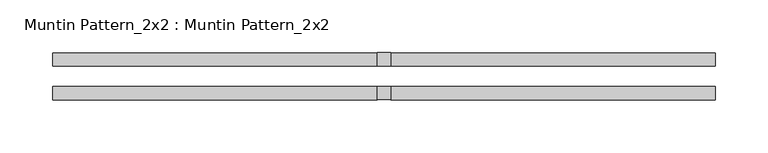
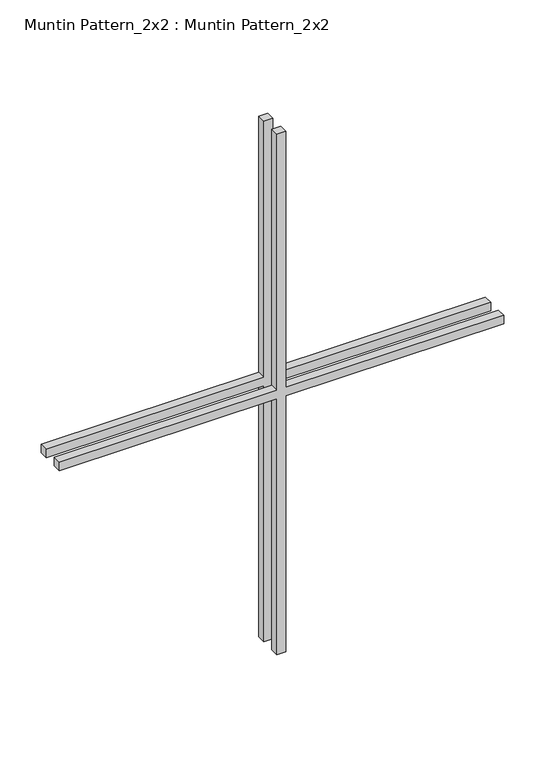
"""IFC4 building model written with IfcOpenShell, lengths in millimetres: proxy geometry, Muntin Pattern_2x2 : Muntin Pattern_2x2."""

from ifc_helpers import new_model, si_unit, frame, origin, place, context, project, spatial, polyline, outline, extrude, source, transform, mapped, element, save


def muntin_pattern_2x2_muntin_pattern_2x2_9352d081(model_context):
    return source(origin(), model_context, "Body", "SweptSolid", [
        extrude(outline(polyline([(393.7, -6.35), (393.7, -312.7375), (381.0, -312.7375), (381.0, -6.35), (0.0, -6.35), (0.0, 6.35), (381.0, 6.35), (381.0, 312.7375), (393.7, 312.7375), (393.7, 6.35), (774.7, 6.35), (774.7, -6.35), (393.7, -6.35)])), frame((0.0, 9.525, 0.0), z_axis=(0.0, 1.0, 0.0), x_axis=(0.0, 0.0, 1.0)), (0.0, 0.0, 1.0), 12.7),
        extrude(outline(polyline([(393.7, -6.35), (393.7, -312.7375), (381.0, -312.7375), (381.0, -6.35), (0.0, -6.35), (0.0, 6.35), (381.0, 6.35), (381.0, 312.7375), (393.7, 312.7375), (393.7, 6.35), (774.7, 6.35), (774.7, -6.35), (393.7, -6.35)])), frame((0.0, -22.225, 0.0), z_axis=(0.0, 1.0, 0.0), x_axis=(0.0, 0.0, 1.0)), (0.0, 0.0, 1.0), 12.7),
    ])


if __name__ == "__main__":
    model = new_model("IFC4")
    model_context = context("Model", 3, world=origin())
    ifc_project = project(units=[si_unit("LENGTHUNIT", "METRE", prefix="MILLI")], contexts=[model_context])
    site = spatial("IfcSite", under=ifc_project)
    building = spatial("IfcBuilding", under=site)
    placement = place(None, origin())
    muntin_pattern_2x2_muntin_pattern_2x2_shape = muntin_pattern_2x2_muntin_pattern_2x2_9352d081(model_context)
    element("IfcBuildingElementProxy", 1, Name="Muntin Pattern_2x2 : Muntin Pattern_2x2", ObjectType="Muntin Pattern_2x2 : Muntin Pattern_2x2", at=placement, inside=building, context=model_context, shape_type="MappedRepresentation", body=[
        mapped(muntin_pattern_2x2_muntin_pattern_2x2_shape, transform((0.0, 0.0, 0.0), x_axis=(1.0, 0.0, 0.0), y_axis=(0.0, 1.0, 0.0), z_axis=(0.0, 0.0, 1.0))),
    ])
    save(model, "model.ifc")

# Revit data of these elements
# Type "Muntin Pattern_2x2 : Muntin Pattern_2x2"
#   Width [instance default] = 4' - 0"
#   Thickness = 0' - 0 1/2"
#   Height [instance default] = 4' - 0"
#   Distance = 0' - 0 3/4"
#   Interior Material [instance default] = none
#   Exterior Material [instance default] = none
#   Default Elevation = 0
# Element 1 (IfcBuildingElementProxy, "Muntin Pattern_2x2 : Muntin Pattern_2x2")
#   Width = 2' - 0 5/8"
#   Height = 2' - 6 1/2"
#   Interior Material = Wood - Stained
#   Exterior Material = Clad - White
#   Materials on its faces: "Clad - White", "Wood - Stained"
# Materials
#   "Clad - White": class "Wood", colour RGB 242 242 238, transparency 0, Cost = 0
#   "Wood - Stained": class "Wood", colour RGB 224 178 126, transparency 0, Cost = 0
